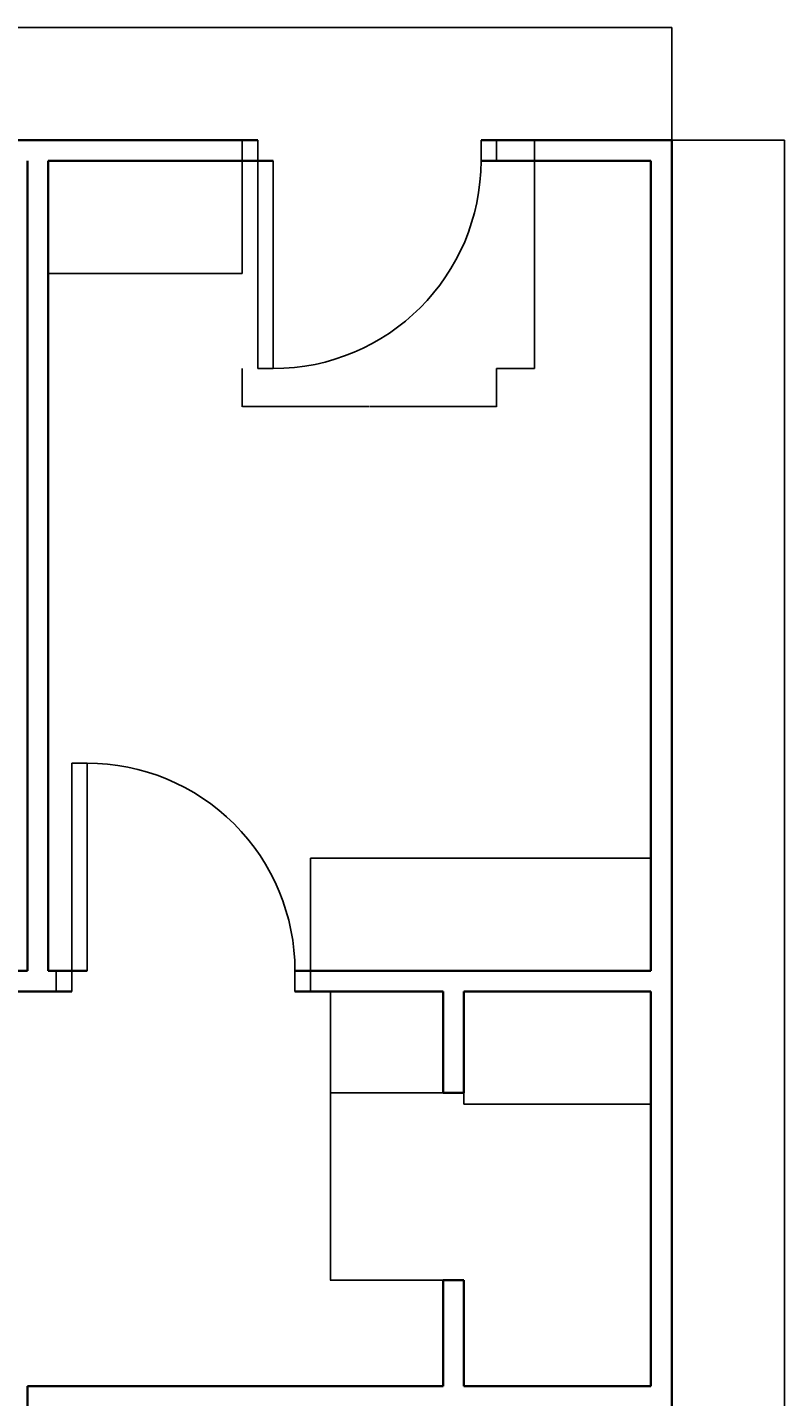
# Model space of a CAD drawing. Units: millimetres. Extents: x 1426 to 11512, y -8522 to 2664.
# Tile 4 of 4: x 7869 to 11512, y -3929 to 2664. Entities that reach past the tile are written whole.
import ezdxf

# ---------------------------------------------------------------- set-up
doc = ezdxf.new("R2010")
doc.units = ezdxf.units.MM
for name, color, linetype, lineweight in [('A-ANNO-DIMS', 2, 'Continuous', 18), ('A-DOOR', 3, 'Continuous', 25), ('A-WALL', 7, 'Continuous', 35)]:
    doc.layers.add(name, color=color, linetype=linetype, lineweight=lineweight)
doc.styles.get("Standard").update_dxf_attribs({"font": 'arial.ttf'})
doc.dimstyles.get("Standard").update_dxf_attribs({"dimtxt": 0.18, "dimasz": 0.18, "dimexe": 0.18, "dimexo": 0.0625, "dimgap": 0.09, "dimtad": 0, "dimtih": 1, "dimtoh": 1, "dimdec": 4, "dimzin": 0, "dimdsep": 46, "dimtxsty": 'Standard', "dimcen": 0.09, "dimadec": 0, "dimazin": 0, "dimtfac": 1, "dimtdec": 4, "dimtofl": 0, "dimtmove": 0, "dimatfit": 3, "dimfxl": 1, "dimtolj": 1, "dimtzin": 0, "dimarcsym": 0})

# ---------------------------------------------------------------- blocks, each defined once
blk = doc.blocks.new('DOOR-SINGLE-1000')
for p, q in [((0, 1000), (0, 1100)), ((0, 1100), (74.2, 1100)), ((74.2, 1100), (74.2, 1000)), ((1148.4, 1000), (1148.4, 1100)), ((1148.4, 1100), (1222.6, 1100)), ((1222.6, 1100), (1222.6, 1000)), ((74.2, 1000), (0, 1000)), ((74.2, 1000), (148.4, 1000)), ((74.2, 0), (74.2, 1000)), ((148.4, 1000), (148.4, 0)), ((1222.6, 1000), (1148.4, 1000)), ((148.4, 0), (74.2, 0))]:
    blk.add_line(p, q)
blk.add_arc((148.4, 1000), 1000, 270, 0)
blk = doc.blocks.new('*D12')
at = {"layer": 'A-ANNO-DIMS', "color": 0, "lineweight": -2, "transparency": 16777216}
for p, q in [((8902.8, 1020.9), (8902.8, 837.4)), ((10125.4, 1020.9), (10125.4, 837.4)), ((8903, 837.6), (9512.5, 837.6)), ((10125.2, 837.6), (9515.6, 837.6))]:
    blk.add_line(p, q, dxfattribs=at)
at = {"layer": 'A-ANNO-DIMS', "color": 0, "transparency": 16777216}
for points in [[(8903, 837.6), (8903, 837.5), (8902.8, 837.6)], [(10125.2, 837.6), (10125.2, 837.5), (10125.4, 837.6)]]:
    blk.add_solid(points, dxfattribs=at)
at = {"layer": 'Defpoints', "color": 0, "transparency": 16777216}
for p in [(8902.8, 1020.9), (10125.4, 1020.9), (10125.4, 837.6)]:
    blk.add_point(p, dxfattribs=at)
at = {"layer": 'A-ANNO-DIMS', "color": 0, "transparency": 16777216, "insert": (9514.1, 837.6), "char_height": 0.18, "attachment_point": 5}
blk.add_mtext('\\A1;SINGLE DOOR 1223 TYP.', dxfattribs=at)
blk = doc.blocks.new('*D13')
at = {"layer": 'A-ANNO-DIMS', "color": 0, "lineweight": -2, "transparency": 16777216}
for p, q in [((10125.4, 2120.9), (10308.9, 2120.9)), ((10308.8, 2120.8), (10308.8, 1571.1)), ((10308.8, 1021.1), (10308.8, 1570.8)), ((10125.4, 1020.9), (10308.9, 1020.9))]:
    blk.add_line(p, q, dxfattribs=at)
at = {"layer": 'A-ANNO-DIMS', "color": 0, "transparency": 16777216}
for points in [[(10308.7, 2120.8), (10308.8, 2120.8), (10308.8, 2120.9)], [(10308.7, 1021.1), (10308.8, 1021.1), (10308.8, 1020.9)]]:
    blk.add_solid(points, dxfattribs=at)
at = {"layer": 'Defpoints', "color": 0, "transparency": 16777216}
for p in [(10125.4, 2120.9), (10308.8, 2120.9), (10125.4, 1020.9)]:
    blk.add_point(p, dxfattribs=at)
at = {"layer": 'A-ANNO-DIMS', "color": 0, "transparency": 16777216, "insert": (10308.8, 1570.9), "char_height": 0.18, "attachment_point": 5}
blk.add_mtext('\\A1;1100 TYP.', dxfattribs=at)
blk = doc.blocks.new('*D38')
at = {"layer": 'A-ANNO-DIMS', "color": 0, "lineweight": -2, "transparency": 16777216}
for p, q in [((10968.9, 2120.9), (11511.6, 2120.9)), ((11511.4, 2120.8), (11511.4, -2928.9)), ((11511.4, -7978.9), (11511.4, -2929.2)), ((10968.9, -7979.1), (11511.6, -7979.1))]:
    blk.add_line(p, q, dxfattribs=at)
at = {"layer": 'A-ANNO-DIMS', "color": 0, "transparency": 16777216}
for points in [[(11511.3, 2120.8), (11511.4, 2120.8), (11511.4, 2120.9)], [(11511.3, -7978.9), (11511.4, -7978.9), (11511.4, -7979.1)]]:
    blk.add_solid(points, dxfattribs=at)
at = {"layer": 'Defpoints', "color": 0, "transparency": 16777216}
for p in [(10968.9, 2120.9), (10968.9, -7979.1), (11511.4, -7979.1)]:
    blk.add_point(p, dxfattribs=at)
at = {"layer": 'A-ANNO-DIMS', "color": 0, "transparency": 16777216, "insert": (11511.4, -2929.1), "char_height": 0.18, "attachment_point": 5}
blk.add_mtext('\\A1;10100', dxfattribs=at)
blk = doc.blocks.new('*D39')
at = {"layer": 'A-ANNO-DIMS', "color": 0, "lineweight": -2, "transparency": 16777216}
for p, q in [((1868.9, 2121), (1868.9, 2663.6)), ((1869.1, 2663.4), (6418.5, 2663.4)), ((10968.7, 2663.4), (6419.2, 2663.4)), ((10968.9, 2121), (10968.9, 2663.6))]:
    blk.add_line(p, q, dxfattribs=at)
at = {"layer": 'A-ANNO-DIMS', "color": 0, "transparency": 16777216}
for points in [[(1869.1, 2663.5), (1869.1, 2663.4), (1868.9, 2663.4)], [(10968.7, 2663.5), (10968.7, 2663.4), (10968.9, 2663.4)]]:
    blk.add_solid(points, dxfattribs=at)
at = {"layer": 'Defpoints', "color": 0, "transparency": 16777216}
for p in [(10968.9, 2663.4), (1868.9, 2120.9), (10968.9, 2120.9)]:
    blk.add_point(p, dxfattribs=at)
at = {"layer": 'A-ANNO-DIMS', "color": 0, "transparency": 16777216, "insert": (6418.9, 2663.4), "char_height": 0.18, "attachment_point": 5}
blk.add_mtext('\\A1;9100', dxfattribs=at)
blk = doc.blocks.new('*D47')
at = {"layer": 'A-ANNO-DIMS', "color": 0, "lineweight": -2, "transparency": 16777216}
for p, q in [((9968.9, -1979.1), (9968.9, -2521.7)), ((10868.9, -1979.1), (10868.9, -2521.7)), ((9969.1, -2521.6), (10418.6, -2521.6)), ((10868.7, -2521.6), (10419.2, -2521.6))]:
    blk.add_line(p, q, dxfattribs=at)
at = {"layer": 'A-ANNO-DIMS', "color": 0, "transparency": 16777216}
for points in [[(9969.1, -2521.5), (9969.1, -2521.6), (9968.9, -2521.6)], [(10868.7, -2521.5), (10868.7, -2521.6), (10868.9, -2521.6)]]:
    blk.add_solid(points, dxfattribs=at)
at = {"layer": 'Defpoints', "color": 0, "transparency": 16777216}
for p in [(9968.9, -1979.1), (10868.9, -1979.1), (9968.9, -2521.6)]:
    blk.add_point(p, dxfattribs=at)
at = {"layer": 'A-ANNO-DIMS', "color": 0, "transparency": 16777216, "insert": (10418.9, -2521.6), "char_height": 0.18, "attachment_point": 5}
blk.add_mtext('\\A1;900', dxfattribs=at)
blk = doc.blocks.new('*D58')
at = {"layer": 'A-ANNO-DIMS', "color": 0, "lineweight": -2, "transparency": 16777216}
for p, q in [((7968.9, 2020.9), (7968.9, 1478.3)), ((8902.8, 2020.9), (8902.8, 1478.3)), ((7969.1, 1478.4), (8435.4, 1478.4)), ((8902.6, 1478.4), (8436.2, 1478.4))]:
    blk.add_line(p, q, dxfattribs=at)
at = {"layer": 'A-ANNO-DIMS', "color": 0, "transparency": 16777216}
for points in [[(7969.1, 1478.5), (7969.1, 1478.4), (7968.9, 1478.4)], [(8902.6, 1478.5), (8902.6, 1478.4), (8902.8, 1478.4)]]:
    blk.add_solid(points, dxfattribs=at)
at = {"layer": 'Defpoints', "color": 0, "transparency": 16777216}
for p in [(7968.9, 2020.9), (8902.8, 2020.9), (7968.9, 1478.4)]:
    blk.add_point(p, dxfattribs=at)
at = {"layer": 'A-ANNO-DIMS', "color": 0, "transparency": 16777216, "insert": (8435.8, 1478.4), "char_height": 0.18, "attachment_point": 5}
blk.add_mtext('\\A1;933.9', dxfattribs=at)
blk = doc.blocks.new('*D67')
at = {"layer": 'A-ANNO-DIMS', "color": 0, "lineweight": -2, "transparency": 16777216}
for p, q in [((9868.8, -2466.1), (9326.2, -2466.1)), ((9326.4, -2466.2), (9326.4, -2917.1)), ((9326.4, -3368.3), (9326.4, -2917.5)), ((9868.8, -3368.5), (9326.2, -3368.5))]:
    blk.add_line(p, q, dxfattribs=at)
at = {"layer": 'A-ANNO-DIMS', "color": 0, "transparency": 16777216}
for points in [[(9326.3, -2466.2), (9326.4, -2466.2), (9326.4, -2466.1)], [(9326.3, -3368.3), (9326.4, -3368.3), (9326.4, -3368.5)]]:
    blk.add_solid(points, dxfattribs=at)
at = {"layer": 'Defpoints', "color": 0, "transparency": 16777216}
for p in [(9326.4, -2466.1), (9868.9, -2466.1), (9868.9, -3368.5)]:
    blk.add_point(p, dxfattribs=at)
at = {"layer": 'A-ANNO-DIMS', "color": 0, "transparency": 16777216, "insert": (9326.4, -2917.3), "char_height": 0.18, "attachment_point": 5}
blk.add_mtext('\\A1;902.4', dxfattribs=at)
blk = doc.blocks.new('*D68')
at = {"layer": 'A-ANNO-DIMS', "color": 0, "lineweight": -2, "transparency": 16777216}
for p, q in [((9868.8, -1979.1), (9326.2, -1979.1)), ((9326.4, -1979.2), (9326.4, -2222.4)), ((9326.4, -2465.9), (9326.4, -2222.7)), ((9868.8, -2466.1), (9326.2, -2466.1))]:
    blk.add_line(p, q, dxfattribs=at)
at = {"layer": 'A-ANNO-DIMS', "color": 0, "transparency": 16777216}
for points in [[(9326.3, -1979.2), (9326.4, -1979.2), (9326.4, -1979.1)], [(9326.3, -2465.9), (9326.4, -2465.9), (9326.4, -2466.1)]]:
    blk.add_solid(points, dxfattribs=at)
at = {"layer": 'Defpoints', "color": 0, "transparency": 16777216}
for p in [(9326.4, -1979.1), (9868.9, -1979.1), (9868.9, -2466.1)]:
    blk.add_point(p, dxfattribs=at)
at = {"layer": 'A-ANNO-DIMS', "color": 0, "transparency": 16777216, "insert": (9326.4, -2222.6), "char_height": 0.18, "attachment_point": 5}
blk.add_mtext('\\A1;487', dxfattribs=at)
blk = doc.blocks.new('*D70')
at = {"layer": 'A-ANNO-DIMS', "color": 0, "lineweight": -2, "transparency": 16777216}
for p, q in [((9230.3, -1879), (9230.3, -1336.4)), ((9230.5, -1336.6), (10049.1, -1336.6)), ((10868.7, -1336.6), (10050, -1336.6)), ((10868.9, -1879), (10868.9, -1336.4))]:
    blk.add_line(p, q, dxfattribs=at)
at = {"layer": 'A-ANNO-DIMS', "color": 0, "transparency": 16777216}
for points in [[(9230.5, -1336.5), (9230.5, -1336.6), (9230.3, -1336.6)], [(10868.7, -1336.5), (10868.7, -1336.6), (10868.9, -1336.6)]]:
    blk.add_solid(points, dxfattribs=at)
at = {"layer": 'Defpoints', "color": 0, "transparency": 16777216}
for p in [(10868.9, -1336.6), (9230.3, -1879.1), (10868.9, -1879.1)]:
    blk.add_point(p, dxfattribs=at)
at = {"layer": 'A-ANNO-DIMS', "color": 0, "transparency": 16777216, "insert": (10049.6, -1336.6), "char_height": 0.18, "attachment_point": 5}
blk.add_mtext('\\A1;1638.6', dxfattribs=at)

msp = doc.modelspace()

# ---------------------------------------------------------------- linework, layer by layer
at = {"layer": 'A-WALL'}
for p, q in [((1868.87, 2120.94), (8976.97, 2120.94)), ((10051.17, 2120.94), (10968.87, 2120.94)), ((10968.87, 2120.94), (10968.87, -7979.06)), ((7868.87, -1879.06), (7868.87, 2020.94)), ((7968.87, -1879.06), (7968.87, 2020.94)), ((7968.87, 2020.94), (9051.17, 2020.94)), ((10051.17, 2020.94), (10868.87, 2020.94)), ((10868.87, 2020.94), (10868.87, -1879.06)), ((7234.46, -1879.06), (7868.87, -1879.06)), ((7968.87, -1879.06), (8156.07, -1879.06)), ((9156.07, -1879.06), (10868.87, -1879.06)), ((7234.46, -1979.06), (8081.87, -1979.06)), ((9156.07, -1979.06), (9868.87, -1979.06)), ((9868.87, -1979.06), (9868.87, -2466.06)), ((9968.87, -1979.06), (9968.87, -2466.06)), ((9968.87, -1979.06), (10868.87, -1979.06)), ((10868.87, -1979.06), (10868.87, -3879.06)), ((9968.87, -2466.06), (9868.87, -2466.06)), ((9868.87, -3368.47), (9968.87, -3368.47)), ((9868.87, -3368.47), (9868.87, -3879.06)), ((9968.87, -3368.47), (9968.87, -3879.06)), ((7868.87, -3979.06), (7868.87, -3879.06)), ((7868.87, -3879.06), (9868.87, -3879.06)), ((9968.87, -3879.06), (10868.87, -3879.06))]:
    msp.add_line(p, q, dxfattribs=at)

# ---------------------------------------------------------------- block references
at = {"layer": 'A-DOOR'}
msp.add_blockref('DOOR-SINGLE-1000', (8902.77, 1020.94), dxfattribs=at)
at = {"layer": 'A-DOOR', "extrusion": (0, 0, -1), "zscale": -1, "rotation": 180}
msp.add_blockref('DOOR-SINGLE-1000', (-8007.67, -879.06), dxfattribs=at)

# ---------------------------------------------------------------- dimensions: what is measured, and where the dimension line sits
at = {"layer": 'A-ANNO-DIMS'}
for base, p1, p2, override, picture, middle in [((10968.87, 2663.44), (1868.87, 2120.94), (10968.87, 2120.94), {"dimdec": 0, "dimlfac": 1, "dimrnd": 0, "dimzin": 0, "dimdsep": 46, "dimlunit": 2}, '*D39', (6418.87, 2663.44)), ((10868.87, -1336.56), (9230.27, -1879.06), (10868.87, -1879.06), {"dimdec": 1, "dimlfac": 1, "dimrnd": 0, "dimzin": 0, "dimdsep": 46, "dimlunit": 2}, '*D70', (10049.57, -1336.56))]:
    dim = msp.add_linear_dim(base=base, p1=p1, p2=p2, dimstyle='Standard', override=override, dxfattribs=at)
    dim.commit()
    dim.dimension.update_dxf_attribs({"geometry": picture, "text_midpoint": middle})
dim = msp.add_linear_dim(base=(10308.76, 2120.94), p1=(10125.37, 1020.94), p2=(10125.37, 2120.94), angle=90, text='<> TYP.', dimstyle='Standard', override={"dimdec": 0, "dimlfac": 1, "dimrnd": 0, "dimzin": 0, "dimdsep": 46, "dimlunit": 2}, dxfattribs=at)
dim.commit()
dim.dimension.update_dxf_attribs({"geometry": '*D13', "text_midpoint": (10308.76, 1570.94)})
for base, p1, p2, angle, override, picture, middle in [((11511.37, -7979.06), (10968.87, 2120.94), (10968.87, -7979.06), 90, {"dimdec": 0, "dimlfac": 1, "dimrnd": 0, "dimzin": 0, "dimdsep": 46, "dimlunit": 2}, '*D38', (11511.37, -2929.06)), ((7968.87, 1478.44), (8902.77, 2020.94), (7968.87, 2020.94), 180, {"dimdec": 1, "dimlfac": 1, "dimrnd": 0, "dimzin": 0, "dimdsep": 46, "dimlunit": 2}, '*D58', (8435.82, 1478.44)), ((9326.37, -1979.06), (9868.87, -2466.06), (9868.87, -1979.06), 90, {"dimdec": 0, "dimlfac": 1, "dimrnd": 0, "dimzin": 0, "dimdsep": 46, "dimlunit": 2}, '*D68', (9326.37, -2222.56)), ((9968.87, -2521.56), (10868.87, -1979.06), (9968.87, -1979.06), 180, {"dimdec": 0, "dimlfac": 1, "dimrnd": 0, "dimzin": 0, "dimdsep": 46, "dimlunit": 2}, '*D47', (10418.87, -2521.56)), ((9326.37, -2466.06), (9868.87, -3368.47), (9868.87, -2466.06), 90, {"dimdec": 1, "dimlfac": 1, "dimrnd": 0, "dimzin": 0, "dimdsep": 46, "dimlunit": 2}, '*D67', (9326.37, -2917.27))]:
    dim = msp.add_linear_dim(base=base, p1=p1, p2=p2, angle=angle, dimstyle='Standard', override=override, dxfattribs=at)
    dim.commit()
    dim.dimension.update_dxf_attribs({"geometry": picture, "text_midpoint": middle})
dim = msp.add_linear_dim(base=(10125.37, 837.55), p1=(8902.77, 1020.94), p2=(10125.37, 1020.94), text='SINGLE DOOR <> TYP.', dimstyle='Standard', override={"dimdec": 0, "dimlfac": 1, "dimrnd": 0, "dimzin": 0, "dimdsep": 46, "dimlunit": 2}, dxfattribs=at)
dim.commit()
dim.dimension.update_dxf_attribs({"geometry": '*D12', "text_midpoint": (9514.07, 837.55)})

doc.saveas('drawing.dxf')
